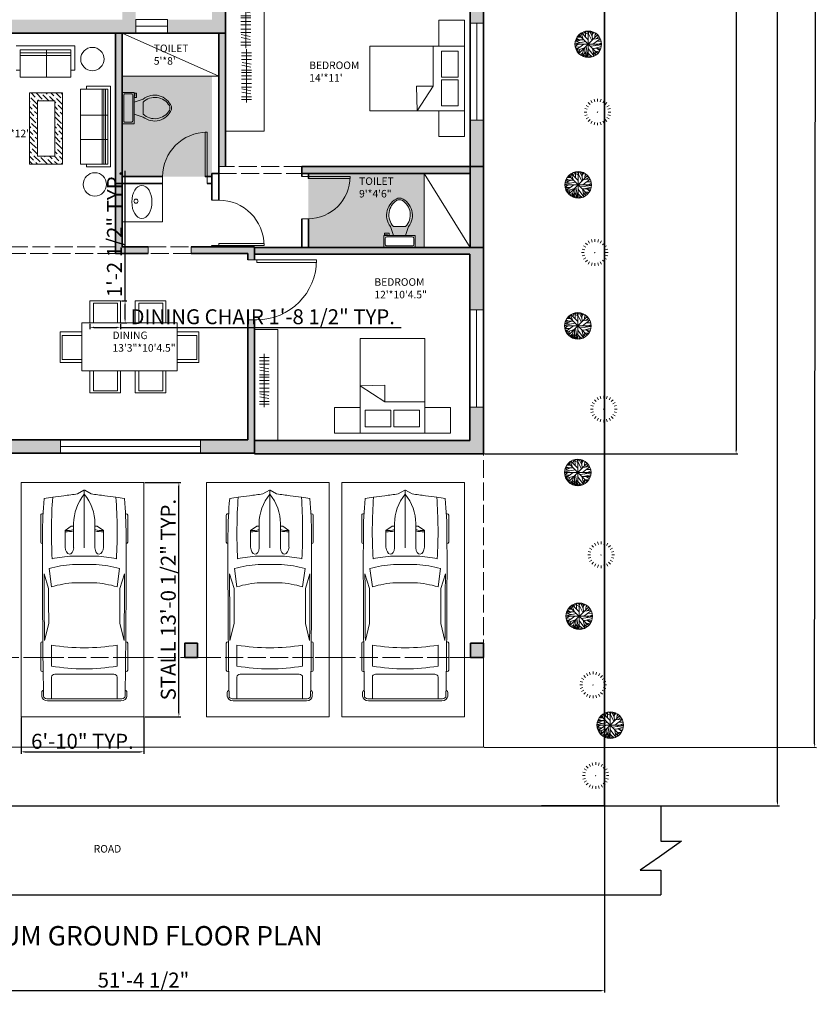
# Model space of a CAD drawing. Units: inches. Extents: x 2852 to 3654, y 1718 to 3031.
# Tile 2 of 5: x 3120 to 3654, y 1718 to 2376. Entities that reach past the tile are written whole.
import ezdxf

# ---------------------------------------------------------------- set-up
doc = ezdxf.new("R2010")
doc.units = ezdxf.units.IN
doc.linetypes.add('ACAD_ISO02W100', pattern=[15, 12, -3])
for name, color, linetype, lineweight in [('A-ANNO-DIMS', 2, 'Continuous', 18), ('A-ANNO-TEXT', 7, 'Continuous', 18), ('A-ANNO-TITL', 7, 'Continuous', 35), ('A-AREA-IDEN', 7, 'Continuous', 18), ('A-COLS', 7, 'Continuous', 35), ('A-COLS-PATT', 8, 'Continuous', 13), ('A-DOOR', 140, 'Continuous', 18), ('A-FLOR-CASE', 210, 'Continuous', 18), ('A-FLOR-FIXT', 9, 'Continuous', 18), ('A-FLOR-PATT', 52, 'Continuous', 13), ('A-FURN-PATT', 210, 'Continuous', 13), ('A-ROOF-OVHD', 140, 'ACAD_ISO02W100', 18), ('A-WALL-OVHD', 140, 'ACAD_ISO02W100', 18), ('A-WALL-PATT', 12, 'Continuous', 13), ('C-PKNG', 8, 'Continuous', 18), ('C-PKNG-VEHI', 140, 'Continuous', 13), ('C-PROP', 7, 'Continuous', 35), ('C-ROAD', 7, 'Continuous', 25), ('fur', 210, 'Continuous', 18), ('tree', 74, 'Continuous', 13), ('wall', 12, 'Continuous', 35), ('window', 140, 'Continuous', 18)]:
    doc.layers.add(name, color=color, linetype=linetype, lineweight=lineweight)
doc.styles.get("Standard").update_dxf_attribs({"font": 'arial.ttf'})
doc.dimstyles.new('ISO-25', dxfattribs={"dimtxt": 10, "dimasz": 2.5, "dimexe": 1.25, "dimexo": 0.625, "dimtad": 1, "dimdec": 0, "dimlunit": 4, "dimtxsty": 'Standard', "dimcen": 2.5, "dimadec": 0, "dimazin": 0, "dimtfac": 1, "dimtdec": 0, "dimtmove": 0, "dimatfit": 3, "dimfxl": 1, "dimarcsym": 0})

# ---------------------------------------------------------------- blocks, each defined once
blk = doc.blocks.new('*U2')
for p, q in [((0, 0), (0, -6)), ((40, 0), (40, -6))]:
    blk.add_line(p, q)
blk.add_lwpolyline([(0, 0), (0, 40), (1.75, 40), (1.75, 0)], close=True)
blk.add_arc((0, 0), 40, 0, 90)
blk = doc.blocks.new('*U6')
for p, q in [((21.1, 37.41), (21.1, 36.83)), ((46.55, 38.89), (22.35, 38.89)), ((47.8, 37.39), (47.8, 37.41)), ((87.99, 31.87), (74.76, 35.92)), ((134.31, 35.6), (119.29, 31.78)), ((135.45, 37.07), (135.45, 37.41)), ((136.7, 38.89), (160.9, 38.89)), ((162.15, 37.41), (162.15, 36.77)), ((70.03, 31.54), (86.41, 29.35)), ((138.42, 29.35), (157.25, 29.35)), ((186.47, 29.35), (167.01, 29.35)), ((186.47, -33.5), (186.47, 33.5)), ((188.4, -32.76), (188.4, 32.76)), ((164.52, 26.39), (164.52, -26.39)), ((29.77, 9.51), (51.68, 9.51)), ((32.12, 9.51), (32.12, 11.15)), ((32.27, 11.63), (36.13, 17.17)), ((36.13, 17.17), (50.94, 17.17)), ((58.92, -10.77), (58.92, 10.77)), ((66.55, -10.53), (66.55, 10.53)), ((186.47, -10.53), (186.47, 10.53)), ((3.27, 6.13), (0.1, 0.41)), ((82.74, 8.5), (82.74, -8.5)), ((0, 0), (51.68, 0)), ((0.1, -0.41), (3.27, -6.13)), ((29.77, -9.51), (51.68, -9.51)), ((32.12, -9.51), (32.12, -11.15)), ((32.27, -11.63), (36.13, -17.17)), ((36.13, -17.17), (50.94, -17.17)), ((86.41, -29.35), (70.03, -31.54)), ((87.99, -31.87), (74.76, -35.92)), ((134.31, -35.6), (119.29, -31.78)), ((157.25, -29.35), (138.42, -29.35)), ((167.01, -29.35), (186.47, -29.35)), ((21.1, -37.41), (21.1, -36.83)), ((46.55, -38.89), (22.35, -38.89)), ((47.8, -37.39), (47.8, -37.41)), ((135.45, -37.07), (135.45, -37.41)), ((136.7, -38.89), (160.9, -38.89)), ((162.15, -37.41), (162.15, -36.77))]:
    blk.add_line(p, q)
for centre, major_axis, ratio, start_param, end_param in [((266.03, -27.52), (0, 313.31), 0.842304, 1.367076, 1.39176), ((41.19, -490.86), (0, 528.23), 0.842304, 0.00281, 0.075598), ((22.35, 37.41), (0, -1.48), 0.842304, 3.141593, 4.712389), ((64.48, -10555.62), (0, 10593.03), 0.842304, -0.013397, 0.002797), ((46.55, 37.41), (0, 1.48), 0.842304, -1.570796, 0), ((64.48, -10555.62), (0, -10591.55), 0.842304, 3.133765, 3.140441), ((136.7, 37.41), (0, -1.48), 0.842304, 3.141593, 4.712389), ((160.9, 37.41), (0, 1.48), 0.842304, -1.570796, 0), ((180.63, 35.84), (0, 2.22), 0.842304, -0.013017, 1.249894), ((64.48, -10556.36), (0, 10595.31), 0.842304, -0.013397, -0.013017), ((183.98, 33.5), (0, -2.96), 0.842304, 1.570796, 3.128196), ((183.98, 32.76), (0, -5.25), 0.842304, 1.570796, 3.128196), ((259.18, -27.52), (0, -305.3), 0.842304, 4.528606, 4.561838), ((37.47, -593.96), (0, -623.33), 0.842304, 3.096046, 3.200911), ((134.4, 5.39), (0, -89.78), 0.842304, 4.449482, 4.652344), ((135.29, 5.39), (0, 81.77), 0.842304, 1.245306, 1.50788), ((149.6, 2.8), (0, -79.58), 0.842304, 4.372215, 4.640744), ((95.79, -3666.35), (0, -3698.24), 0.842304, 3.134049, 3.144098), ((17.08, 0), (0, 147.02), 0.842304, 4.511394, 4.913384), ((35.91, 0), (0, 147.02), 0.842304, 4.511394, 4.913384), ((167.01, 26.39), (0, 2.96), 0.842304, 0, 1.570796), ((-204.49, 52.4), (0, -250.96), 0.842304, 1.385369, 1.434372), ((29.77, -46.66), (0, 56.17), 0.842304, 0, 0.590319), ((32.75, 11.15), (0, 0.74), 0.842304, 0.879714, 1.570796), ((13.04, 17.01), (0, 27.42), 0.842304, 4.435146, 4.718221), ((14.2, 17.01), (0, 27.42), 0.842304, 4.435146, 4.718221), ((50.79, 13.34), (6.34, -0.36), 0.603834, -1.395552, 1.581315), ((0.62, 0), (0, -0.74), 0.842304, 4.131459, 5.293319), ((-204.49, -52.4), (0, 250.96), 0.842304, -1.434372, -1.385369), ((29.77, 46.66), (0, 56.17), 0.842304, 2.551274, 3.141593), ((149.6, -2.8), (0, -79.58), 0.842304, -1.499151, -1.230623), ((32.75, -11.15), (0, -0.74), 0.842304, 4.712389, 5.403472), ((13.04, -17.01), (0, -27.42), 0.842304, 1.564964, 1.848039), ((14.2, -17.01), (0, -27.42), 0.842304, 1.564964, 1.848039), ((134.4, -5.39), (0, -89.78), 0.842304, -1.510751, -1.307889), ((135.29, -5.39), (0, -81.77), 0.842304, -1.50788, -1.245306), ((259.18, 27.52), (0, 305.3), 0.842304, 1.721348, 1.754579), ((167.01, -26.39), (0, -2.96), 0.842304, 4.712389, 6.283185), ((266.03, 27.52), (0, 313.31), 0.842304, 1.749832, 1.774517), ((37.47, 593.96), (0, -623.33), 0.842304, -0.059319, 0.045547), ((95.79, 3666.35), (0, -3698.24), 0.842304, -0.002505, 0.007544), ((183.98, -33.5), (0, 2.96), 0.842304, 3.15499, 4.712389), ((183.98, -32.76), (0, -5.25), 0.842304, 0.013397, 1.570796), ((41.19, 490.86), (0, -528.23), 0.842304, -0.075598, -0.00281), ((22.35, -37.41), (0, 1.48), 0.842304, 1.570796, 3.141593), ((64.48, 10555.62), (0, 10593.03), 0.842304, 3.138796, 3.15499), ((46.55, -37.41), (0, -1.48), 0.842304, 0, 1.570796), ((64.48, 10555.62), (0, -10591.55), 0.842304, 0.001152, 0.007828), ((136.7, -37.41), (0, -1.48), 0.842304, -1.570796, 0), ((160.9, -37.41), (0, 1.48), 0.842304, 3.141593, 4.712389), ((180.63, -35.84), (0, -2.22), 0.842304, -1.249894, 0.013017), ((64.48, 10556.36), (0, 10595.31), 0.842304, 3.15461, 3.15499)]:
    blk.add_ellipse(centre, major_axis=major_axis, ratio=ratio, start_param=start_param, end_param=end_param)
at = {"extrusion": (0, 0, -1)}
blk.add_ellipse((50.79, -13.34), major_axis=(6.34, 0.36), ratio=0.603834, start_param=-1.395552, end_param=1.581315, dxfattribs=at)
blk = doc.blocks.new('*U4')
for p, q in [((9.5, -6), (9.5, -2)), ((-10, -8.5), (-8, -8.5)), ((-10, -9.5), (-10, -8.5)), ((-7, -9.5), (-10, -9.5)), ((-8, -8.5), (-8, -8)), ((-7, -8), (-7, -9.5)), ((-4, -8), (-6, -14)), ((4, -8), (6, -14)), ((4, -14), (-4, -14))]:
    blk.add_line(p, q)
blk.add_lwpolyline([(10.5, -8), (10.5, 0), (-10.5, 0), (-10.5, -8)], close=True)
for points in [[(-9.5, -2), (-9.5, -6)], [(8.5, -1), (-8.5, -1)], [(-8.5, -7), (8.5, -7)]]:
    blk.add_lwpolyline(points)
for centre, radius, start, end in [((-8.62, -1.88), 0.884, 81.8699, 188.1301), ((-8.62, -6.12), 0.884, 171.8699, 278.1301), ((8.62, -1.88), 0.884, 351.8699, 98.1301), ((8.62, -6.12), 0.884, 261.8699, 8.1301), ((3.52, -21.58), 12.17, 141.46911, 247.97143), ((4.2, -21.82), 11.33, 136.36773, 238.94682), ((-3.52, -21.58), 12.17, 292.02843, 38.53071), ((-4.2, -21.82), 11.33, 301.05301, 43.63209), ((0, -27.88), 4, 245.73182, 294.26817), ((0, -29), 4, 254.86053, 285.13947)]:
    blk.add_arc(centre, radius, start, end)
blk = doc.blocks.new('*U10')
for p, q in [((-40.1797, 44.558), (-36.4825, 43.2038)), ((-37.0107, 47.0408), (-35.25, 35.5298)), ((-32.6092, 50.4264), (-23.2782, 23.5674)), ((-31.2008, 51.1035), (-0.2149, 20.1818)), ((-26.4472, 46.5894), (-26.2712, 53.8116)), ((-22.0458, 42.0753), (-16.5881, 57.6486)), ((-21.1656, 55.8436), (-0.0388, 45.0094)), ((-12.5388, 54.9406), (-7.9613, 59.4546)), ((-12.3627, 32.1443), (-12.5388, 58.7776)), ((-5.3205, 59.6806), (16.5105, 16.7963)), ((2.426, 54.9406), (-1.4472, 59.9056)), ((0, 59.9996), (0, -60)), ((0.4894, 48.6208), (3.6584, 59.6806)), ((18.2711, 35.5298), (5.419, 59.6806)), ((9.8203, 51.5549), (12.8133, 58.5516)), ((19.6795, 19.5047), (16.3344, 57.6486)), ((17.0387, 51.1035), (23.2006, 55.1666)), ((17.7429, 43.6552), (25.4894, 54.2636)), ((31.6513, 50.8778), (30.2429, 30.5643)), ((31.1232, 42.5267), (35.8767, 48.1693)), ((-59.7219, 2.8025), (-12.0106, 12.0565)), ((-32.2571, 20.6333), (-59.1937, 9.348)), ((-58.6656, 12.7336), (-35.9543, 7.5424)), ((-57.081, 17.9248), (-47.0458, 14.7649)), ((-56.0247, 20.859), (-20.8134, 20.859)), ((-54.7923, 24.4702), (-47.75, 21.0847)), ((-54.6162, -24.7335), (-20.2853, 0.0941)), ((-53.2078, 27.4044), (-40.1797, 20.859)), ((-49.8627, 32.8214), (-32.7853, 32.8214)), ((-45.8134, 38.2383), (-40.5318, 33.0471)), ((-43.8768, 36.4326), (-44.405, 40.2696)), ((42, 42), (-42, -42)), ((42, -42), (-42, 42)), ((54.3626, 25.3731), (20.9119, 0.3198)), ((23.3767, 23.3417), (53.3063, 27.4044)), ((29.3626, -6.6771), (59.4682, 7.091)), ((36.2288, 25.1474), (48.9049, 35.0784)), ((37.1091, 37.1098), (46.6161, 37.5612)), ((38.5175, 13.4107), (58.2359, 13.6364)), ((-60, 0), (60, 0)), ((-59.7219, -4.8714), (-54.2641, -6.6771)), ((-45.2853, -0.1316), (-59.0177, -10.0627)), ((-58.4895, -12.3197), (-36.4825, -11.6426)), ((-57.081, -18.4138), (-45.2853, -17.9624)), ((-52.6797, -18.188), (-55.4966, -22.0251)), ((-53.2078, -27.442), (-16.7641, -16.6081)), ((-38.9472, -29.0219), (-51.4472, -30.6018)), ((-47.2219, -19.3166), (-50.2148, -26.3135)), ((-46.5177, -30.1504), (-49.5106, -33.536)), ((-32.4331, -32.4075), (-48.1021, -35.5674)), ((-43.7008, -34.6645), (-46.6937, -37.373)), ((-35.9543, -22.4765), (-44.0529, -40.5329)), ((-24.6867, -37.8244), (-38.7712, -45.7241)), ((-26.2712, -43.9185), (-34.7219, -48.6583)), ((-19.9331, -20.2194), (-28.5599, -52.721)), ((-14.6515, -36.2445), (-27.6797, -52.9467)), ((-14.8275, -15.0282), (-14.6515, -57.6865)), ((-14.6515, -32.1818), (-3.912, -59.4922)), ((-10.074, -10.0627), (-2.5036, -59.7178)), ((-6.2008, -36.2445), (17.919, -57.0094)), ((-0.0388, -19.0909), (25.8415, -53.8495)), ((9.2922, -9.1598), (59.6443, -2.8401)), ((18.6232, -18.6394), (26.7218, -53.3981)), ((18.7992, -18.6394), (57.3556, -17.2853)), ((22.8485, -36.4702), (35.3485, -48.4326)), ((26.3697, -18.4138), (58.9401, -9.8369)), ((30.419, -30.1504), (32.3556, -50.0125)), ((31.4753, -31.279), (49.6091, -33.3103)), ((38.1654, -18.188), (52.426, -29.0219)), ((41.5105, -32.6332), (46.088, -38.0501)), ((45.9119, -24.0564), (55.595, -22.2508)), ((-14.6515, -47.3041), (-25.0388, -54.3009)), ((-21.5177, -45.4984), (-19.9331, -56.1065)), ((-8.4895, -47.5298), (-11.4825, -58.5893)), ((-6.3768, -52.721), (-9.3698, -58.815)), ((8.4119, -53.1724), (3.8344, -59.4922)), ((5.9471, -46.6269), (10.5246, -58.5893)), ((24.7852, -44.8213), (23.0246, -54.978))]:
    blk.add_line(p, q)
blk.add_circle((0, 0), 60)
blk = doc.blocks.new('*U9')
for p, q in [((-25.024, 42.079), (-31.077, 52.563)), ((-13.435, 46.72), (-16.606, 58.557)), ((-1.077, 60.601), (-1.077, 48.601)), ((11.28, 46.72), (14.452, 58.557)), ((22.87, 42.079), (28.923, 52.563)), ((-61.077, 0.601), (-49.077, 0.601)), ((-47.5, 13.04), (-59.033, 16.131)), ((-42.564, 24.554), (-53.039, 30.601)), ((-34.93, 34.454), (-43.503, 43.028)), ((32.776, 34.454), (41.349, 43.028)), ((40.409, 24.554), (50.884, 30.601)), ((45.346, 13.04), (56.878, 16.131)), ((58.923, 0.601), (46.923, 0.601)), ((-47.5, -11.837), (-59.033, -14.928)), ((-42.564, -23.351), (-53.039, -29.399)), ((-34.93, -33.251), (-43.503, -41.825)), ((-25.024, -40.876), (-31.077, -51.36)), ((22.87, -40.876), (28.923, -51.36)), ((32.776, -33.251), (41.349, -41.825)), ((40.409, -23.351), (50.884, -29.399)), ((45.346, -11.837), (56.878, -14.928)), ((-13.435, -45.517), (-16.606, -57.354)), ((-1.077, -59.399), (-1.077, -47.399)), ((11.28, -45.517), (14.452, -57.354))]:
    blk.add_line(p, q)
blk.add_lwpolyline([(-1.908, 0.978), (-2.67, -0.978), (0, 0)], close=True)
blk = doc.blocks.new('*D12')
at = {"layer": 'A-ANNO-DIMS', "color": 0, "lineweight": -2, "transparency": 16777216}
for p, q in [((3430.58, 2927.69), (3600.09, 2927.69)), ((3598.84, 2925.19), (3598.84, 2088.69)), ((3430.58, 2086.19), (3600.09, 2086.19))]:
    blk.add_line(p, q, dxfattribs=at)
at = {"layer": 'A-ANNO-DIMS', "color": 0, "lineweight": 100, "transparency": 16777216}
for points in [[(3598.42, 2925.19), (3599.25, 2925.19), (3598.84, 2927.69)], [(3598.42, 2088.69), (3599.25, 2088.69), (3598.84, 2086.19)]]:
    blk.add_solid(points, dxfattribs=at)
at = {"layer": 'Defpoints', "color": 0, "lineweight": 100, "transparency": 16777216}
for p in [(3429.95, 2927.69), (3429.95, 2086.19), (3598.84, 2086.19)]:
    blk.add_point(p, dxfattribs=at)
at = {"layer": 'A-ANNO-DIMS', "color": 0, "transparency": 16777216, "insert": (3593.1, 2506.94), "char_height": 10, "attachment_point": 5, "rotation": 90}
blk.add_mtext('70\'-2"', dxfattribs=at)
blk = doc.blocks.new('*D13')
at = {"layer": 'A-ANNO-DIMS', "color": 0, "lineweight": -2, "transparency": 16777216}
for p, q in [((3431.69, 2930.92), (3653.8, 2930.67)), ((3651.35, 1892.32), (3652.54, 2928.17)), ((3430.49, 1890.07), (3652.6, 1889.82))]:
    blk.add_line(p, q, dxfattribs=at)
at = {"layer": 'A-ANNO-DIMS', "color": 0, "lineweight": 100, "transparency": 16777216}
for points in [[(3652.13, 2928.17), (3652.96, 2928.17), (3652.55, 2930.67)], [(3650.94, 1892.32), (3651.77, 1892.32), (3651.35, 1889.82)]]:
    blk.add_solid(points, dxfattribs=at)
at = {"layer": 'Defpoints', "color": 0, "lineweight": 100, "transparency": 16777216}
for p in [(3431.06, 2930.92), (3652.55, 2930.67), (3429.87, 1890.07)]:
    blk.add_point(p, dxfattribs=at)
at = {"layer": 'A-ANNO-DIMS', "color": 0, "transparency": 16777216, "insert": (3646.22, 2410.25), "char_height": 10, "attachment_point": 5, "rotation": 89.93413}
blk.add_mtext('86\'-9"', dxfattribs=at)
blk = doc.blocks.new('BED-WITH-NIGHTSTANDS')
for p, q in [((42.38, 60.42), (42.38, 33.67)), ((42.38, 33.67), (31.23, 33.67)), ((31.23, 33.67), (31.64, 17.23)), ((31.64, 17.23), (42.38, 33.67))]:
    blk.add_line(p, q)
for points in [[(63.28, 60.42), (46.24, 60.42), (46.24, 77.65), (63.28, 77.65)], [(63.28, 60.42), (0, 60.42), (0, 17.23), (63.28, 17.23)], [(59.11, 57), (47.96, 57), (47.96, 39.69), (59.11, 39.69)], [(59.11, 37.81), (47.96, 37.81), (47.96, 20.49), (59.11, 20.49)], [(63.28, 0), (46.24, 0), (46.24, 17.23), (63.28, 17.23)]]:
    blk.add_lwpolyline(points, close=True)
blk = doc.blocks.new('WARDROBE-HANGING-RAIL')
for p, q in [((0, 3.21), (35.71, 3.21)), ((2.45, 0), (2.45, 6.54)), ((4.63, 0), (4.63, 6.54)), ((6.93, 0), (6.93, 6.54)), ((8.87, 0.34), (10.08, 6.34)), ((10.83, 0.21), (12.05, 6.21)), ((14.06, 0), (14.06, 6.54)), ((15.59, 0), (15.59, 6.54)), ((17.86, 0), (17.86, 6.54)), ((20.11, 0), (20.11, 6.54)), ((23.04, 0), (23.04, 6.54)), ((25.39, 0), (25.39, 6.54)), ((26.68, 0.21), (27.9, 6.21)), ((28.71, 0.21), (29.93, 6.21)), ((31.85, 0), (31.85, 6.54)), ((33.7, 0), (33.7, 6.54))]:
    blk.add_line(p, q)
blk = doc.blocks.new('CHAIR-DINING')
for p, q in [((0, 0), (0, 14.57)), ((0, 14.57), (20.41, 14.57)), ((20.41, 14.57), (20.41, 0))]:
    blk.add_line(p, q)
blk.add_lwpolyline([(2.32, 0), (18.35, 0), (18.35, 13.17), (2.32, 13.17)], close=True)
blk = doc.blocks.new('ROAD-BREAK')
for p, q in [((13.81, 59.39), (13.81, 35.82)), ((27.65, 35.82), (12.74, 25.36)), ((13.81, 35.82), (27.65, 35.82)), ((12.74, 25.36), (0, 16.42)), ((0, 16.42), (13.81, 16.42)), ((13.81, 16.42), (13.81, 0))]:
    blk.add_line(p, q)
blk = doc.blocks.new('PARKING-STALL')
blk.add_lwpolyline([(0, 156.52), (82.03, 156.52), (82.03, 0), (0, 0)], close=True)
blk = doc.blocks.new('*D27')
at = {"layer": 'A-ANNO-DIMS', "color": 0, "lineweight": -2, "transparency": 16777216}
for p, q in [((3166.9, 2173.19), (3166.9, 2169.5)), ((3187.31, 2173.19), (3187.31, 2169.5)), ((3169.4, 2170.75), (3184.81, 2170.75)), ((3187.31, 2170.75), (3374.94, 2170.75))]:
    blk.add_line(p, q, dxfattribs=at)
at = {"layer": 'A-ANNO-DIMS', "color": 0, "lineweight": 100, "transparency": 16777216}
for points in [[(3169.4, 2171.17), (3169.4, 2170.33), (3166.9, 2170.75)], [(3184.81, 2171.17), (3184.81, 2170.33), (3187.31, 2170.75)]]:
    blk.add_solid(points, dxfattribs=at)
at = {"layer": 'Defpoints', "color": 0, "lineweight": 100, "transparency": 16777216}
for p in [(3166.9, 2173.81), (3187.31, 2173.81), (3187.31, 2170.75)]:
    blk.add_point(p, dxfattribs=at)
at = {"layer": 'A-ANNO-DIMS', "color": 0, "transparency": 16777216, "insert": (3282.37, 2176.55), "char_height": 10, "attachment_point": 5}
blk.add_mtext('DINING CHAIR 1\'-8 1/2" TYP.', dxfattribs=at)
blk = doc.blocks.new('*D28')
at = {"layer": 'A-ANNO-DIMS', "color": 0, "lineweight": -2, "transparency": 16777216}
for p, q in [((3190.37, 2188.38), (3190.37, 2275.44)), ((3187.93, 2188.38), (3191.62, 2188.38)), ((3190.37, 2176.31), (3190.37, 2185.88)), ((3187.93, 2173.81), (3191.62, 2173.81))]:
    blk.add_line(p, q, dxfattribs=at)
at = {"layer": 'A-ANNO-DIMS', "color": 0, "lineweight": 100, "transparency": 16777216}
for points in [[(3189.95, 2185.88), (3190.78, 2185.88), (3190.37, 2188.38)], [(3189.95, 2176.31), (3190.78, 2176.31), (3190.37, 2173.81)]]:
    blk.add_solid(points, dxfattribs=at)
at = {"layer": 'Defpoints', "color": 0, "lineweight": 100, "transparency": 16777216}
for p in [(3187.31, 2188.38), (3190.37, 2188.38), (3187.31, 2173.81)]:
    blk.add_point(p, dxfattribs=at)
at = {"layer": 'A-ANNO-DIMS', "color": 0, "transparency": 16777216, "insert": (3184.57, 2233.16), "char_height": 10, "attachment_point": 5, "rotation": 90}
blk.add_mtext('1\'-2 1/2" TYP.', dxfattribs=at)
blk = doc.blocks.new('*D35')
at = {"layer": 'A-ANNO-DIMS', "color": 0, "lineweight": -2, "transparency": 16777216}
for p, q in [((3203.48, 2067.03), (3227.58, 2067.03)), ((3226.33, 1913.01), (3226.33, 2064.53)), ((3203.48, 1910.51), (3227.58, 1910.51))]:
    blk.add_line(p, q, dxfattribs=at)
at = {"layer": 'A-ANNO-DIMS', "color": 0, "lineweight": 100, "transparency": 16777216}
for points in [[(3225.91, 2064.53), (3226.75, 2064.53), (3226.33, 2067.03)], [(3225.91, 1913.01), (3226.75, 1913.01), (3226.33, 1910.51)]]:
    blk.add_solid(points, dxfattribs=at)
at = {"layer": 'Defpoints', "color": 0, "lineweight": 100, "transparency": 16777216}
for p in [(3202.85, 2067.03), (3226.33, 2067.03), (3202.85, 1910.51)]:
    blk.add_point(p, dxfattribs=at)
at = {"layer": 'A-ANNO-DIMS', "color": 0, "transparency": 16777216, "insert": (3220.53, 1988.77), "char_height": 10, "attachment_point": 5, "rotation": 90}
blk.add_mtext('STALL 13\'-0 1/2" TYP.', dxfattribs=at)
blk = doc.blocks.new('*D36')
at = {"layer": 'A-ANNO-DIMS', "color": 0, "lineweight": -2, "transparency": 16777216}
for p, q in [((3120.82, 1909.89), (3120.82, 1885.78)), ((3202.85, 1909.89), (3202.85, 1885.78)), ((3123.32, 1887.03), (3200.35, 1887.03))]:
    blk.add_line(p, q, dxfattribs=at)
at = {"layer": 'A-ANNO-DIMS', "color": 0, "lineweight": 100, "transparency": 16777216}
for points in [[(3123.32, 1887.45), (3123.32, 1886.62), (3120.82, 1887.03)], [(3200.35, 1887.45), (3200.35, 1886.62), (3202.85, 1887.03)]]:
    blk.add_solid(points, dxfattribs=at)
at = {"layer": 'Defpoints', "color": 0, "lineweight": 100, "transparency": 16777216}
for p in [(3120.82, 1910.51), (3202.85, 1910.51), (3202.85, 1887.03)]:
    blk.add_point(p, dxfattribs=at)
at = {"layer": 'A-ANNO-DIMS', "color": 0, "transparency": 16777216, "insert": (3161.84, 1892.77), "char_height": 10, "attachment_point": 5}
blk.add_mtext('6\'-10" TYP.', dxfattribs=at)
blk = doc.blocks.new('*D39')
at = {"layer": 'A-ANNO-DIMS', "color": 0, "lineweight": -2, "transparency": 16777216}
for p, q in [((2894.37, 1850.19), (2894.37, 1726.13)), ((3510.95, 1850.19), (3510.95, 1726.13)), ((2896.87, 1727.38), (3508.45, 1727.38))]:
    blk.add_line(p, q, dxfattribs=at)
at = {"layer": 'A-ANNO-DIMS', "color": 0, "lineweight": 100, "transparency": 16777216}
for points in [[(2896.87, 1727.79), (2896.87, 1726.96), (2894.37, 1727.38)], [(3508.45, 1727.79), (3508.45, 1726.96), (3510.95, 1727.38)]]:
    blk.add_solid(points, dxfattribs=at)
at = {"layer": 'Defpoints', "color": 0, "lineweight": 100, "transparency": 16777216}
for p in [(2894.37, 1850.82), (3510.95, 1850.82), (3510.95, 1727.38)]:
    blk.add_point(p, dxfattribs=at)
at = {"layer": 'A-ANNO-DIMS', "color": 0, "transparency": 16777216, "insert": (3202.66, 1733.17), "char_height": 10, "attachment_point": 5}
blk.add_mtext('51\'-4 1/2"', dxfattribs=at)
blk = doc.blocks.new('*D40')
at = {"layer": 'A-ANNO-DIMS', "color": 0, "lineweight": -2, "transparency": 16777216}
for p, q in [((3511.58, 2951.69), (3627.74, 2951.69)), ((3626.49, 1853.32), (3626.49, 2949.19)), ((3511.58, 1850.82), (3627.74, 1850.82))]:
    blk.add_line(p, q, dxfattribs=at)
at = {"layer": 'A-ANNO-DIMS', "color": 0, "lineweight": 100, "transparency": 16777216}
for points in [[(3626.07, 2949.19), (3626.9, 2949.19), (3626.49, 2951.69)], [(3626.07, 1853.32), (3626.9, 1853.32), (3626.49, 1850.82)]]:
    blk.add_solid(points, dxfattribs=at)
at = {"layer": 'Defpoints', "color": 0, "lineweight": 100, "transparency": 16777216}
for p in [(3510.95, 2951.69), (3626.49, 2951.69), (3510.95, 1850.82)]:
    blk.add_point(p, dxfattribs=at)
at = {"layer": 'A-ANNO-DIMS', "color": 0, "transparency": 16777216, "insert": (3620.76, 2401.26), "char_height": 10, "attachment_point": 5, "rotation": 90}
blk.add_mtext('91\'-9"', dxfattribs=at)

msp = doc.modelspace()

# ---------------------------------------------------------------- hatches: boundary and pattern name
at = {"layer": 'A-COLS-PATT'}
h = msp.add_hatch(color=256, dxfattribs=at)
h.dxf.hatch_style = 1
h.paths.add_polyline_path([(2950.9, 1959.59), (2942.37, 1959.59), (2942.37, 1950.07), (2950.9, 1950.07)])
h.paths.add_polyline_path([(3107.14, 1959.59), (3098.61, 1959.59), (3098.61, 1950.07), (3107.14, 1950.07)])
h.paths.add_polyline_path([(3238.77, 1959.59), (3230.24, 1959.59), (3230.24, 1950.07), (3238.77, 1950.07)])
h.paths.add_polyline_path([(3429.87, 1959.59), (3421.34, 1959.59), (3421.34, 1950.07), (3429.87, 1950.07)])
at = {"layer": 'A-FLOR-PATT'}
h = msp.add_hatch(dxfattribs=at)
h.set_pattern_fill('ANGLE', color=256)
h.set_pattern_definition([(0, (0, 0), (0, 6.985), [5.08, -1.905]), (90, (0, 0), (-6.985, 4e-16), [5.08, -1.905])])
h.paths.add_polyline_path([(3248.45, 2849.58), (3188.45, 2849.58), (3188.45, 2844.77), (3196.45, 2844.77), (3196.45, 2842.27), (3196.95, 2842.27), (3196.95, 2844.27), (3197.95, 2844.27), (3197.95, 2841.27), (3196.45, 2841.27), (3196.45, 2838.27), (3202.45, 2840.27, -0.501317), (3221.31, 2835.31, -0.132891), (3221.31, 2833.22, -0.501323), (3202.45, 2828.27), (3196.45, 2830.27), (3196.45, 2823.77), (3188.45, 2823.77), (3188.45, 2783.69), (3215.78, 2783.69), (3215.78, 2783.73, -0.401453), (3244.71, 2813.96), (3244.71, 2813.99), (3246.03, 2813.99), (3246.03, 2783.69), (3248.45, 2783.69)])
h.paths.add_polyline_path([(3420.95, 2714.69), (3324.42, 2714.69), (3324.42, 2691.18, -1), (3301.33, 2691.18), (3301.33, 2638.19), (3420.95, 2638.19)])
h.paths.add_polyline_path([(3059.57, 2647.05, -0.132891), (3061.66, 2647.05, -0.501323), (3066.62, 2628.19), (3064.62, 2622.19), (3071.12, 2622.19), (3071.12, 2614.19), (3084.95, 2614.19), (3084.95, 2678.69), (3040.14, 2678.69), (3040.14, 2677.19), (3040.14, 2637.19), (3038.39, 2637.19), (3038.39, 2637.23, -0.401453), (3000.14, 2677.19), (3000.14, 2678.69), (2994.25, 2678.69), (2994.25, 2614.19), (3050.12, 2614.19), (3050.12, 2622.19), (3052.62, 2622.19), (3052.62, 2622.69), (3050.62, 2622.69), (3050.62, 2623.69), (3053.62, 2623.69), (3053.62, 2622.19), (3056.62, 2622.19), (3054.62, 2628.19, -0.501317)])
h.paths.add_polyline_path([(3252.95, 2533.88, -0.400409), (3223.79, 2561.89), (3223.76, 2561.89), (3223.76, 2563.17), (3252.95, 2563.17), (3252.95, 2565.48), (3192.95, 2565.48), (3192.95, 2500.92), (3252.95, 2500.92)])
h.paths.add_polyline_path([(3248.45, 2338.72), (3188.45, 2338.72), (3188.45, 2271.48), (3248.45, 2271.48), (3248.45, 2273.69)])
h.paths.add_polyline_path([(3390.34, 2273.69), (3312.95, 2273.69), (3312.95, 2224.19), (3390.34, 2224.19)])
h.paths.add_polyline_path([(3365.33, 2231.19), (3382.33, 2231.19, -0.5), (3383.33, 2230.19), (3383.33, 2226.19, -0.5), (3382.33, 2225.19), (3365.33, 2225.19, -0.5), (3364.33, 2226.19), (3364.33, 2230.19, -0.5)], flags=16)
h.paths.add_polyline_path([(3372.19, 2255.72, -0.215004), (3375.48, 2255.72, -0.48008), (3377.83, 2238.19), (3369.83, 2238.19, -0.48008)], flags=16)
h.paths.add_polyline_path([(2987.37, 2220.07), (2951.37, 2220.07), (2951.37, 2095.57), (2987.37, 2095.57)])
at = {"layer": 'A-FURN-PATT'}
h = msp.add_hatch(dxfattribs=at)
h.set_pattern_fill('ANSI36', color=256, scale=0.741806, angle=90)
h.set_pattern_definition([(135, (5014.7031, 0.534), (-4.5798562, 1.2490517), [5.888086, -1.1776172, 0, -1.1776172])])
h.paths.add_polyline_path([(3148.6, 2279.81), (3148.6, 2327.41), (3126.43, 2327.41), (3126.43, 2279.81)])
h.paths.add_polyline_path([(3131.73, 2285.11), (3131.73, 2322.11), (3143.3, 2322.11), (3143.3, 2285.11)], flags=16)
at = {"layer": 'A-WALL-PATT'}
h = msp.add_hatch(color=256, dxfattribs=at)
h.dxf.hatch_style = 1
h.paths.add_polyline_path([(2952.95, 2875.19), (2957.35, 2875.19), (2957.35, 2877.98), (2957.35, 2884.19), (2943.95, 2884.19), (2942.37, 2884.19), (2942.37, 2849.42), (2952.95, 2849.42)])
h.paths.add_polyline_path([(2952.95, 2706.39), (2952.95, 2749.45), (2942.37, 2749.45), (2942.37, 2667.89), (2952.95, 2667.89), (2952.95, 2678.69), (3000.14, 2678.69), (3000.14, 2683.19), (2952.95, 2683.19)])
h.paths.add_polyline_path([(2951.37, 2609.69), (3089.45, 2609.69), (3089.45, 2683.19), (3089.45, 2685.28), (3084.95, 2685.28), (3084.95, 2683.19), (3084.95, 2614.19), (2952.95, 2614.19), (2952.95, 2625.26), (2942.37, 2625.26), (2942.37, 2588.19), (2951.37, 2588.19)])
h.paths.add_polyline_path([(2951.37, 2506.48), (2951.37, 2523.26), (2942.37, 2523.26), (2942.37, 2465.69), (2951.37, 2465.69), (2951.37, 2466.48)])
h.paths.add_polyline_path([(2951.37, 2367.57), (2951.37, 2370.4), (2951.37, 2376.57), (2942.37, 2376.57), (2942.37, 2312.8), (2951.37, 2312.8), (2951.37, 2320.57), (2951.37, 2324.07)])
h.paths.add_polyline_path([(3051.87, 2324.07), (3047.37, 2324.07), (2951.37, 2324.07), (2951.37, 2320.57), (3047.37, 2320.57), (3047.37, 2296.57), (3047.37, 2266.82), (3051.87, 2266.82)])
h.paths.add_polyline_path([(2951.37, 2224.57), (2942.37, 2224.57), (2942.37, 2186.63), (2951.37, 2186.63), (2951.37, 2220.07)])
h.paths.add_polyline_path([(2951.37, 2247.87), (2942.37, 2247.87), (2942.37, 2224.57), (2951.37, 2224.57)])
h.paths.add_polyline_path([(3113.37, 2224.57), (2951.37, 2224.57), (2951.37, 2220.07), (3113.37, 2220.07)])
h.paths.add_polyline_path([(2951.37, 2121.7), (2942.37, 2121.7), (2942.37, 2086.57), (3113.37, 2086.57), (3147.16, 2086.57), (3147.16, 2095.57), (3113.37, 2095.57), (2951.37, 2095.57)])
h.paths.add_polyline_path([(3429.87, 2224.19), (3276.87, 2224.19), (3276.87, 2219.69), (3420.87, 2219.69), (3420.87, 2182.43), (3429.87, 2182.43)])
h.paths.add_polyline_path([(3276.87, 2175.85), (3272.37, 2175.85), (3272.37, 2095.57), (3240.86, 2095.57), (3240.86, 2086.57), (3276.87, 2086.57)])
h.paths.add_polyline_path([(3276.87, 2224.57), (3234.52, 2224.57), (3234.52, 2220.07), (3272.37, 2220.07), (3272.37, 2215.85), (3276.87, 2215.85)])
h = msp.add_hatch(color=256, dxfattribs=at)
h.dxf.hatch_style = 1
h.paths.add_polyline_path([(3188.45, 2266.98), (3183.95, 2266.98), (3183.95, 2224.57), (3183.95, 2220.07), (3205.81, 2220.07), (3205.81, 2224.57), (3188.45, 2224.57)])
h.paths.add_polyline_path([(3188.45, 2367.48), (3183.95, 2367.48), (3183.95, 2266.98), (3188.45, 2266.98), (3188.45, 2271.48)])
h.paths.add_polyline_path([(3051.87, 2376.48), (3017.1, 2376.48), (3017.1, 2372.85), (3017.1, 2367.57), (3047.37, 2367.57), (3051.87, 2367.57), (3051.87, 2372.07)])
h.paths.add_polyline_path([(3197.45, 2376.48), (3197.45, 2460.48), (3225.82, 2460.48), (3225.82, 2469.48), (3188.45, 2469.48), (3188.45, 2376.48), (3051.87, 2376.48), (3051.87, 2372.07), (3051.87, 2367.48), (3197.45, 2367.48)])
h.paths.add_polyline_path([(3257.45, 2410.19), (3257.45, 2469.48), (3247.17, 2469.48), (3247.17, 2460.48), (3248.45, 2460.48), (3248.45, 2376.48), (3218.8, 2376.48), (3218.8, 2367.48), (3257.45, 2367.48)])
h.paths.add_polyline_path([(3257.45, 2367.48), (3252.95, 2367.48), (3252.95, 2278.19), (3257.45, 2278.19)])
h.paths.add_polyline_path([(3420.95, 2278.19), (3308.45, 2278.19), (3308.45, 2273.69), (3420.95, 2273.69)])
h.paths.add_polyline_path([(3257.45, 2527.51), (3257.45, 2533.88), (3252.95, 2533.88), (3252.95, 2469.48), (3257.45, 2469.48)])
h.paths.add_polyline_path([(3257.45, 2609.69), (3259.24, 2609.69), (3259.24, 2614.19), (3252.95, 2614.19), (3227.77, 2614.19), (3227.77, 2611.84), (3227.77, 2609.69), (3252.95, 2609.69), (3252.95, 2563.17), (3253.06, 2563.17), (3257.45, 2563.17)])
h.paths.add_polyline_path([(3196.43, 2614.19), (3188.45, 2614.19), (3188.45, 2569.84), (3188.45, 2469.48), (3192.95, 2469.48), (3192.95, 2565.48), (3252.95, 2565.48), (3252.95, 2569.98), (3192.95, 2569.98), (3192.95, 2609.69), (3196.43, 2609.69), (3196.43, 2611.84)])
h = msp.add_hatch(color=256, dxfattribs=at)
h.dxf.hatch_style = 1
h.paths.add_polyline_path([(3429.87, 2117.5), (3420.87, 2117.5), (3420.87, 2095.19), (3276.87, 2095.19), (3276.87, 2086.19), (3429.87, 2086.19)])
h.paths.add_polyline_path([(3429.95, 2278.19), (3420.95, 2278.19), (3420.95, 2273.69), (3420.95, 2224.19), (3429.95, 2224.19)])
h.paths.add_polyline_path([(3429.95, 2309.24), (3420.95, 2309.24), (3420.95, 2278.19), (3429.95, 2278.19)])
h.paths.add_polyline_path([(3429.95, 2419.19), (3420.95, 2419.19), (3420.95, 2410.19), (3420.95, 2374.17), (3429.95, 2374.17)])
h.paths.add_polyline_path([(3429.95, 2478.26), (3420.95, 2478.26), (3420.95, 2419.19), (3429.95, 2419.19)])
h.paths.add_polyline_path([(3420.95, 2419.19), (3257.45, 2419.19), (3257.45, 2410.19), (3283.32, 2410.19), (3420.95, 2410.19)])

# ---------------------------------------------------------------- linework, layer by layer
at = {"layer": 'A-COLS'}
msp.add_line((3429.87, 1950.07), (3429.87, 1959.59), dxfattribs=at)
for points in [[(3230.24, 1950.07), (3238.77, 1950.07), (3238.77, 1959.59), (3230.24, 1959.59)], [(3421.34, 1950.07), (3429.87, 1950.07), (3429.87, 1959.59), (3421.34, 1959.59)]]:
    msp.add_lwpolyline(points, close=True, dxfattribs=at)
at = {"layer": 'A-FLOR-CASE'}
for points in [[(3257.45, 2301.87), (3283.32, 2301.87), (3283.32, 2410.19), (3257.45, 2410.19)], [(3276.87, 2095.19), (3292.47, 2095.19), (3292.47, 2169.23), (3276.87, 2169.23)]]:
    msp.add_lwpolyline(points, close=True, dxfattribs=at)
at = {"layer": 'A-FLOR-FIXT'}
for p, q in [((3252.95, 2338.72), (3188.45, 2367.48)), ((3188.45, 2338.72), (3248.45, 2338.72)), ((3248.45, 2338.72), (3252.95, 2338.72)), ((3390.34, 2224.19), (3390.34, 2273.69)), ((3390.34, 2273.69), (3420.95, 2224.19)), ((3215.45, 2266.98), (3215.45, 2241.21)), ((3215.45, 2241.21), (3188.45, 2241.21))]:
    msp.add_line(p, q, dxfattribs=at)
msp.add_lwpolyline([(3390.34, 2224.19), (3420.95, 2224.19), (3420.95, 2273.69), (3390.34, 2273.69)], close=True, dxfattribs=at)
msp.add_circle((3197.63, 2255.11), 1.4, dxfattribs=at)
msp.add_ellipse((3201.6, 2254.58), major_axis=(0, 10.98), ratio=0.61364, dxfattribs=at)
at = {"layer": 'A-ROOF-OVHD'}
for p, q in [((3429.87, 1950.07), (3429.87, 2086.19)), ((2942.37, 1950.07), (3429.87, 1950.07))]:
    msp.add_line(p, q, dxfattribs=at)
at = {"layer": 'A-WALL-OVHD'}
for p, q in [((3205.81, 2224.57), (3205.81, 2220.07)), ((3234.52, 2224.57), (3234.52, 2220.07))]:
    msp.add_line(p, q, dxfattribs=at)
for points in [[(3308.45, 2278.19), (3252.95, 2278.19), (3252.95, 2273.69), (3308.45, 2273.69)], [(3113.37, 2224.57), (3183.95, 2224.57), (3183.95, 2220.07), (3113.37, 2220.07)], [(3205.81, 2224.57), (3234.52, 2224.57), (3234.52, 2220.07), (3205.81, 2220.07)]]:
    msp.add_lwpolyline(points, close=True, dxfattribs=at)
at = {"layer": 'C-PKNG'}
for p, q in [((3134.03, 1950.07), (3141.16, 1950.07)), ((3185.06, 1950.07), (3202.85, 1950.07)), ((3230.24, 1950.07), (3244.82, 1950.07)), ((3258.03, 1950.07), (3265.16, 1950.07)), ((3309.06, 1950.07), (3316.19, 1950.07)), ((3326.85, 1950.07), (3335.32, 1950.07)), ((3348.53, 1950.07), (3355.66, 1950.07)), ((3399.56, 1950.07), (3406.69, 1950.07)), ((3417.35, 1950.07), (3429.87, 1950.07)), ((3429.87, 1890.07), (3429.87, 1950.07)), ((2942.37, 1890.07), (3429.87, 1890.07))]:
    msp.add_line(p, q, dxfattribs=at)
at = {"layer": 'C-PROP'}
for p, q in [((3510.95, 2951.69), (3510.95, 1890.07)), ((3510.95, 1890.07), (3510.95, 1850.82)), ((3510.95, 1850.82), (3468.85, 1850.82))]:
    msp.add_line(p, q, dxfattribs=at)
at = {"layer": 'C-ROAD'}
for p, q in [((2910.23, 1850.82), (3468.85, 1850.82)), ((3468.85, 1850.82), (3548.59, 1850.82)), ((2910.23, 1791.43), (3468.85, 1791.43)), ((3468.85, 1791.43), (3548.59, 1791.43))]:
    msp.add_line(p, q, dxfattribs=at)
at = {"layer": 'fur'}
for p, q in [((3117.65, 2358.82), (3156.83, 2358.82)), ((3120.33, 2356.22), (3154.07, 2356.22)), ((3137.82, 2356.22), (3137.82, 2337.9)), ((3154.07, 2356.22), (3154.07, 2337.9)), ((3156.83, 2358.82), (3156.83, 2342.6)), ((3120.33, 2354.35), (3154.07, 2354.35)), ((3120.33, 2352.39), (3154.07, 2352.39)), ((3120.33, 2342.6), (3117.65, 2342.6)), ((3156.83, 2342.6), (3154.07, 2342.6)), ((3180.55, 2331.91), (3164.55, 2331.91)), ((3164.55, 2331.91), (3164.55, 2329.97)), ((3175.11, 2279.8), (3175.11, 2329.97)), ((3176.24, 2279.8), (3176.24, 2329.97)), ((3177.34, 2279.8), (3177.34, 2329.97)), ((3180.55, 2277.97), (3180.55, 2331.91)), ((3178.86, 2312.48), (3160.54, 2312.48)), ((3178.86, 2296.22), (3160.54, 2296.22)), ((3164.55, 2279.8), (3164.55, 2277.97)), ((3164.55, 2277.97), (3180.55, 2277.97))]:
    msp.add_line(p, q, dxfattribs=at)
msp.add_lwpolyline([(3154.07, 2356.22), (3120.33, 2356.22), (3120.33, 2337.9), (3154.07, 2337.9)], dxfattribs=at)
for points in [[(3178.86, 2279.8), (3178.86, 2329.97), (3160.54, 2329.97), (3160.54, 2279.8)], [(3148.6, 2279.81), (3148.6, 2327.41), (3126.43, 2327.41), (3126.43, 2279.81)], [(3143.3, 2285.11), (3143.3, 2322.11), (3131.73, 2322.11), (3131.73, 2285.11)], [(3161.56, 2173.81), (3225.15, 2173.81), (3225.15, 2141.59), (3161.56, 2141.59)]]:
    msp.add_lwpolyline(points, close=True, dxfattribs=at)
for centre in [(3168.5, 2350.11), (3170.16, 2266.32)]:
    msp.add_circle(centre, 7.79, dxfattribs=at)
at = {"layer": 'wall'}
for p, q in [((3257.45, 2367.48), (3257.45, 2469.48)), ((3429.95, 2278.19), (3429.95, 2419.19)), ((3420.95, 2278.19), (3420.95, 2410.19)), ((3051.87, 2367.48), (3248.45, 2367.48)), ((3183.95, 2367.48), (3183.95, 2266.98)), ((3257.45, 2367.48), (3188.45, 2367.48)), ((3188.45, 2367.48), (3188.45, 2271.48)), ((3252.95, 2367.48), (3252.95, 2273.69)), ((3257.45, 2367.48), (3257.45, 2278.19)), ((3252.95, 2278.19), (3252.95, 2255.81)), ((3429.95, 2278.19), (3308.45, 2278.19)), ((3308.45, 2278.19), (3308.45, 2271.48)), ((3308.45, 2278.19), (3400.58, 2278.19)), ((3420.95, 2273.69), (3420.95, 2278.19)), ((3429.95, 2224.19), (3429.95, 2278.19)), ((3188.45, 2271.48), (3215.45, 2271.48)), ((3188.45, 2271.48), (3188.45, 2224.57)), ((3243.87, 2271.48), (3248.45, 2271.48)), ((3248.45, 2273.69), (3248.45, 2255.81)), ((3252.95, 2273.69), (3248.45, 2273.69)), ((3420.95, 2273.69), (3308.45, 2273.69)), ((3312.95, 2273.69), (3312.95, 2270.25)), ((3420.95, 2224.19), (3420.95, 2273.69)), ((3183.95, 2266.98), (3215.45, 2266.98)), ((3183.95, 2266.98), (3183.95, 2224.57)), ((3245.17, 2266.98), (3248.45, 2266.98)), ((3308.45, 2243.38), (3308.45, 2224.19)), ((3312.95, 2243.38), (3312.95, 2224.19)), ((3183.95, 2224.57), (3183.95, 2220.07)), ((3205.81, 2224.57), (3188.45, 2224.57)), ((3276.87, 2224.57), (3234.52, 2224.57)), ((3248.45, 2225.55), (3248.45, 2224.57)), ((3252.95, 2225.55), (3252.95, 2224.57)), ((3276.87, 2215.85), (3276.87, 2224.57)), ((3205.81, 2220.07), (3183.95, 2220.07)), ((3272.37, 2220.07), (3234.52, 2220.07)), ((3272.37, 2215.85), (3272.37, 2220.07)), ((3429.87, 2224.19), (3276.87, 2224.19)), ((3420.87, 2219.69), (3276.87, 2219.69)), ((3420.87, 2095.19), (3420.87, 2219.69)), ((3429.87, 2086.19), (3429.87, 2224.19)), ((3272.37, 2095.57), (3272.37, 2175.85)), ((3276.87, 2086.57), (3276.87, 2175.85)), ((3113.37, 2095.57), (3272.37, 2095.57)), ((3276.87, 2095.19), (3420.87, 2095.19)), ((3113.37, 2086.57), (3276.87, 2086.57)), ((3276.87, 2086.19), (3429.87, 2086.19))]:
    msp.add_line(p, q, dxfattribs=at)
at = {"layer": 'window'}
for p, q in [((3197.45, 2371.98), (3218.8, 2371.98)), ((3425.45, 2309.24), (3425.45, 2374.17)), ((3425.37, 2117.5), (3425.37, 2182.43)), ((3147.16, 2091.07), (3240.86, 2091.07))]:
    msp.add_line(p, q, dxfattribs=at)
for points in [[(3197.45, 2376.48), (3218.8, 2376.48), (3218.8, 2367.48), (3197.45, 2367.48)], [(3420.95, 2374.17), (3429.95, 2374.17), (3429.95, 2309.24), (3420.95, 2309.24)], [(3420.87, 2182.43), (3429.87, 2182.43), (3429.87, 2117.5), (3420.87, 2117.5)], [(3147.16, 2095.57), (3240.86, 2095.57), (3240.86, 2086.57), (3147.16, 2086.57)]]:
    msp.add_lwpolyline(points, close=True, dxfattribs=at)

# ---------------------------------------------------------------- block references
at = {"layer": 'A-DOOR', "xscale": -0.7431328879607847, "yscale": 0.7431328879607847, "zscale": 0.7431328879607847}
msp.add_blockref('*U2', (3245.17, 2271.44), dxfattribs=at)
at = {"layer": 'A-DOOR', "rotation": 270}
for p, xscale, yscale, zscale in [((3312.67, 2271.48), 0.7025818617498685, 0.7025818617498685, 0.7025818617498685), ((3252.99, 2225.55), -0.7565136894284056, 0.7565136894284056, 0.7565136894284056)]:
    msp.add_blockref('*U2', p, dxfattribs=dict(at, xscale=xscale, yscale=yscale, zscale=zscale))
msp.add_blockref('*U2', (3278.37, 2215.85), dxfattribs=at)
at = {"layer": 'A-FLOR-CASE'}
for p, rotation in [((3267.8, 2393.13), 270.0000000000057), ((3268.3, 2356.77), 270), ((3280.15, 2153.05), 270)]:
    msp.add_blockref('WARDROBE-HANGING-RAIL', p, dxfattribs=dict(at, rotation=rotation))
at = {"layer": 'A-FLOR-FIXT', "xscale": -1}
for p, rotation in [((3188.45, 2317.33), 90), ((3373.83, 2224.19), 180)]:
    msp.add_blockref('*U4', p, dxfattribs=dict(at, rotation=rotation))
at = {"layer": 'C-PKNG'}
for p in [(3120.82, 1910.51), (3244.82, 1910.51), (3335.32, 1910.51)]:
    msp.add_blockref('PARKING-STALL', p, dxfattribs=at)
at = {"layer": 'C-PKNG-VEHI', "xscale": 0.7477922120772245, "yscale": 0.7477922120772245, "zscale": 0.7477922120772245, "rotation": 270}
for p in [(3163.11, 2061.92), (3287.11, 2061.92), (3377.61, 2061.92)]:
    msp.add_blockref('*U6', p, dxfattribs=at)
at = {"layer": 'C-ROAD'}
msp.add_blockref('ROAD-BREAK', (3534.79, 1791.43), dxfattribs=at)
at = {"layer": 'fur'}
for name, p in [('BED-WITH-NIGHTSTANDS', (3353.95, 2298.33)), ('CHAIR-DINING', (3166.9, 2173.81)), ('CHAIR-DINING', (3197.15, 2173.81))]:
    msp.add_blockref(name, p, dxfattribs=at)
at = {"layer": 'fur', "extrusion": (0, 0, -1), "zscale": -1}
for p, rotation in [((-3161.56, 2167.7), 270.0000000000032), ((-3166.9, 2141.59), 180), ((-3197.15, 2141.59), 180)]:
    msp.add_blockref('CHAIR-DINING', p, dxfattribs=dict(at, rotation=rotation))
at = {"layer": 'fur'}
for name, p, rotation in [('CHAIR-DINING', (3225.15, 2167.7), 270.0000000000017), ('BED-WITH-NIGHTSTANDS', (3330.28, 2163.41), 270.0000000000011)]:
    msp.add_blockref(name, p, dxfattribs=dict(at, rotation=rotation))
at = {"layer": 'tree', "xscale": 0.1480989313836924, "yscale": 0.1480989313836924, "zscale": 0.1480989313836924}
for name, p in [('*U10', (3500.02, 2359.96)), ('*U9', (3506.4, 2314.59)), ('*U10', (3493.3, 2266)), ('*U9', (3504.64, 2220.7)), ('*U10', (3493.04, 2171.71)), ('*U9', (3510.51, 2116.04)), ('*U10', (3492.98, 2073.72)), ('*U9', (3508.74, 2018.65)), ('*U10', (3493.95, 1977.61)), ('*U9', (3503.38, 1931.67)), ('*U10', (3514.72, 1904.87)), ('*U9', (3505.14, 1871.06))]:
    msp.add_blockref(name, p, dxfattribs=at)

# ---------------------------------------------------------------- texts
at = {"layer": 'A-ANNO-TEXT', "insert": (3169.4, 1824.72), "char_height": 5.041, "attachment_point": 1}
msp.add_mtext_dynamic_manual_height_columns('ROAD', width=98.3816, gutter_width=25.21, heights=[0], dxfattribs=at)
at = {"layer": 'A-ANNO-TITL', "insert": (3055.38, 1770.57), "char_height": 12.998, "attachment_point": 1}
msp.add_mtext_dynamic_manual_height_columns('SITE CUM GROUND FLOOR PLAN', width=2588.4992, gutter_width=64.99, heights=[0], dxfattribs=at)
at = {"layer": 'A-AREA-IDEN', "attachment_point": 1}
for s, insert, char_height in [("TOILET\\P5'*8'", (3209.57, 2359.76), 5.041), ("BEDROOM\\P14'*11'", (3313.49, 2348.43), 5.041), ('LIVING\\P10\'10.5"*12\'', (3087.23, 2311.26), 5.0412), ('TOILET\\P9\'*4\'6"', (3346.8, 2271.01), 5.041), ('BEDROOM\\P12\'*10\'4.5"', (3357.05, 2203.57), 5.0412), ('DINING\\P13\'3"*10\'4.5"', (3181.97, 2167.93), 5.0412)]:
    msp.add_mtext_dynamic_manual_height_columns(s, width=98.3816, gutter_width=25.21, heights=[0], dxfattribs=dict(at, insert=insert, char_height=char_height))

# ---------------------------------------------------------------- dimensions: what is measured, and where the dimension line sits
at = {"layer": 'A-ANNO-DIMS'}
for base, p1, p2, override, picture, middle in [((3626.49, 2951.69), (3510.95, 1850.82), (3510.95, 2951.69), {"dimdec": 1, "dimlfac": 1, "dimrnd": 0, "dimzin": 1, "dimdsep": 46, "dimlunit": 4, "dimfrac": 2}, '*D40', (3620.76, 2401.26)), ((3598.8351856, 2086.1927699), (3429.95105595, 2927.6927699), (3429.95105595, 2086.1927699), {"dimclrd": 0, "dimclre": 0, "dimclrt": 0}, '*D12', (3593.10445572, 2506.9427699))]:
    dim = msp.add_linear_dim(base=base, p1=p1, p2=p2, angle=90, dimstyle='ISO-25', override=override, dxfattribs=at)
    dim.commit()
    dim.dimension.update_dxf_attribs({"geometry": picture, "text_midpoint": middle})
dim = msp.add_aligned_dim(p1=(3429.87, 1890.07), p2=(3431.06, 2930.92), distance=-221.48, dimstyle='ISO-25', override={"dimclrd": 0, "dimclre": 0, "dimclrt": 0}, dxfattribs=at)
dim.commit()
dim.dimension.update_dxf_attribs({"geometry": '*D13', "text_midpoint": (3646.22, 2410.25)})
for base, p1, p2, text, picture, middle in [((3190.37, 2188.38), (3187.31, 2173.81), (3187.31, 2188.38), '<> TYP.', '*D28', (3184.57, 2233.16)), ((3226.33, 2067.03), (3202.85, 1910.51), (3202.85, 2067.03), 'STALL <> TYP.', '*D35', (3220.53, 1988.77))]:
    dim = msp.add_linear_dim(base=base, p1=p1, p2=p2, angle=90, text=text, dimstyle='ISO-25', override={"dimdec": 1, "dimlfac": 1, "dimrnd": 0, "dimzin": 1, "dimdsep": 46, "dimlunit": 4, "dimfrac": 2}, dxfattribs=at)
    dim.commit()
    dim.dimension.update_dxf_attribs({"geometry": picture, "text_midpoint": middle})
for base, p1, p2, text, picture, middle in [((3187.31, 2170.75), (3166.9, 2173.81), (3187.31, 2173.81), 'DINING CHAIR <> TYP.', '*D27', (3282.37, 2176.55)), ((3202.85, 1887.03), (3120.82, 1910.51), (3202.85, 1910.51), '<> TYP.', '*D36', (3161.84, 1892.77))]:
    dim = msp.add_linear_dim(base=base, p1=p1, p2=p2, text=text, dimstyle='ISO-25', override={"dimdec": 1, "dimlfac": 1, "dimrnd": 0, "dimzin": 1, "dimdsep": 46, "dimlunit": 4, "dimfrac": 2}, dxfattribs=at)
    dim.commit()
    dim.dimension.update_dxf_attribs({"geometry": picture, "text_midpoint": middle})
dim = msp.add_linear_dim(base=(3510.95, 1727.38), p1=(2894.37, 1850.82), p2=(3510.95, 1850.82), dimstyle='ISO-25', override={"dimdec": 1, "dimlfac": 1, "dimrnd": 0, "dimzin": 1, "dimdsep": 46, "dimlunit": 4, "dimfrac": 2}, dxfattribs=at)
dim.commit()
dim.dimension.update_dxf_attribs({"geometry": '*D39', "text_midpoint": (3202.66, 1733.17)})

doc.saveas('drawing.dxf')
